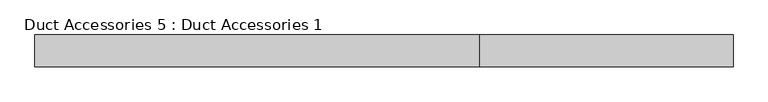
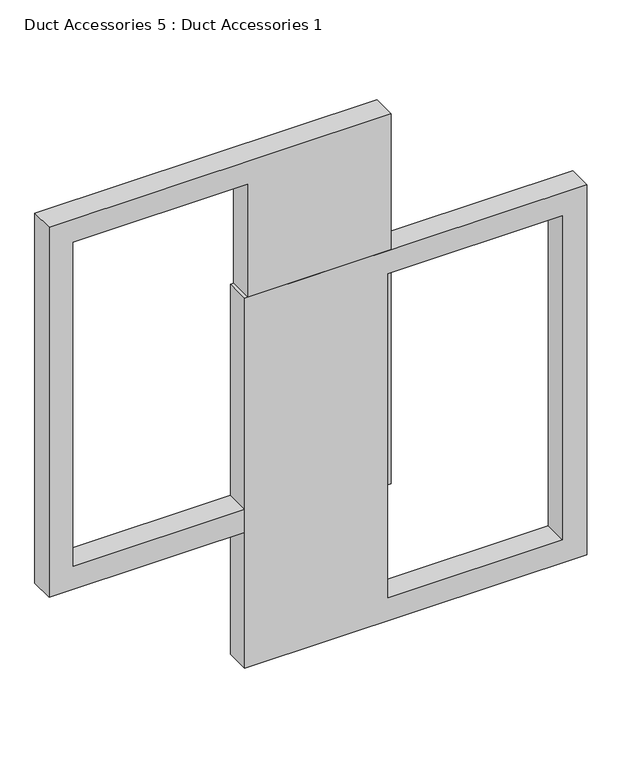
"""IFC4 building model written with IfcOpenShell, lengths in millimetres: damper geometry, Duct Accessories 5 : Duct Accessories 1."""

from ifc_helpers import new_model, si_unit, frame, origin, place, context, project, spatial, polyline, outline, extrude, source, transform, mapped, element, save


def duct_accessories_5_duct_accessories_1_bcda36b2(model_context):
    return source(origin(), model_context, "Body", "SweptSolid", [
        extrude(outline(polyline([(26030.7403114, -12928.36893), (24811.5403114, -12928.36893), (24811.5403114, -11861.56893), (26030.7403114, -11861.56893), (26030.7403114, -12928.36893)]), holes=[polyline([(25954.5403114, -12480.9324751), (25954.5403114, -11937.76893), (24887.7403114, -11937.76893), (24887.7403114, -12480.9324751), (25954.5403114, -12480.9324751)])]), frame((0.0, -447.4934478, 0.0), z_axis=(0.0, 1.0, 0.0), x_axis=(0.0, 0.0, 1.0)), (0.0, 0.0, 1.0), 76.2),
        extrude(outline(polyline([(26478.1767663, -12471.5606701), (26478.1767663, -13538.3606701), (25258.9767663, -13538.3606701), (25258.9767663, -12471.5606701), (26478.1767663, -12471.5606701)]), holes=[polyline([(26401.9767663, -12918.997125), (25335.1767663, -12918.997125), (25335.1767663, -13462.1606701), (26401.9767663, -13462.1606701), (26401.9767663, -12918.997125)])]), frame((0.0, -447.4934478, 0.0), z_axis=(0.0, 1.0, 0.0), x_axis=(0.0, 0.0, 1.0)), (0.0, 0.0, 1.0), 76.2),
    ])


if __name__ == "__main__":
    model = new_model("IFC4")
    model_context = context("Model", 3, world=origin())
    ifc_project = project(units=[si_unit("LENGTHUNIT", "METRE", prefix="MILLI")], contexts=[model_context])
    site = spatial("IfcSite", under=ifc_project)
    building = spatial("IfcBuilding", under=site)
    placement = place(None, origin())
    duct_accessories_5_duct_accessories_1_shape = duct_accessories_5_duct_accessories_1_bcda36b2(model_context)
    element("IfcDamper", 1, ObjectType="Duct Accessories 5 : Duct Accessories 1", at=placement, inside=building, context=model_context, shape_type="MappedRepresentation", body=[
        mapped(duct_accessories_5_duct_accessories_1_shape, transform((0.0, 0.0, 0.0), x_axis=(1.0, 0.0, 0.0), y_axis=(0.0, 1.0, 0.0), z_axis=(0.0, 0.0, 1.0))),
    ])
    save(model, "model.ifc")

# Revit data of these elements
# Element 1 (IfcDamper, "Duct Accessories 5 : Duct Accessories 1")
#   Materials on its faces: "border"
# Materials
#   "border": class "Generic", colour RGB 144 144 144, transparency 0, Cost = 0
